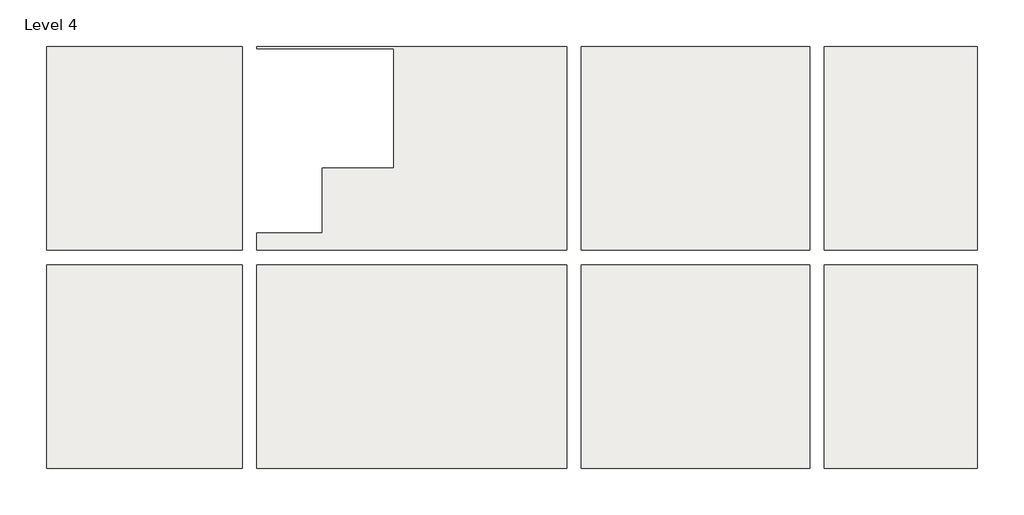
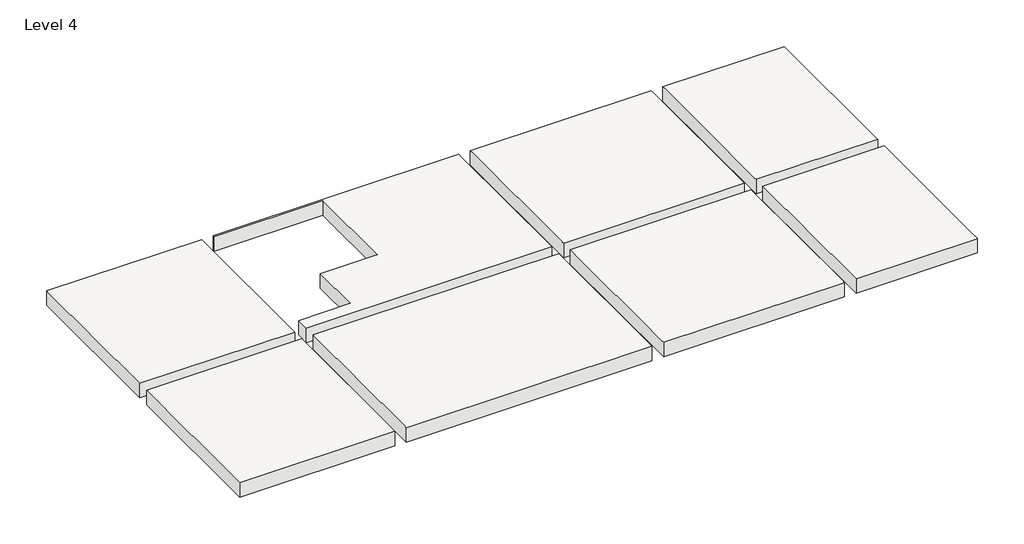
# One storey: 2 slabs.
"""IFC4 building model written with IfcOpenShell, lengths in millimetres."""

from ifc_helpers import new_model, si_unit, origin, place, context, project, spatial, faceted_brep, element, save

model = new_model("IFC4")

# Units and contexts
model_context = context("Model", 3, world=origin())
ifc_project = project(units=[si_unit("LENGTHUNIT", "METRE", prefix="MILLI")], contexts=[model_context])

# Site, building, storey
site = spatial("IfcSite", under=ifc_project)
building = spatial("IfcBuilding", under=site)
storey = spatial("IfcBuildingStorey", under=building, Name="Level 4", Elevation=6048.0)

# Slabs
placement = place(None, origin())
element("IfcSlab", 1, ObjectType="Generic 300mm", at=placement, inside=storey, context=model_context, shape_type="Brep", body=[
    faceted_brep([(-2066.1068817, 2270.4765586, 5700.0), (-5114.1068817, 2270.4765586, 5700.0), (-5114.1068817, 5445.3180792, 5700.0), (-2066.1068817, 5445.3180792, 5700.0), (-2066.1068817, 2270.4765586, 6000.0), (-2066.1068817, 2346.6765586, 6000.0), (-2066.1068817, 5407.2180792, 6000.0), (-2066.1068817, 5445.3180792, 6000.0), (-5114.1068817, 5445.3180792, 6000.0), (-5114.1068817, 5407.2180792, 6000.0), (-5114.1068817, 2346.6765586, 6000.0), (-5114.1068817, 2270.4765586, 6000.0)], [[[0, 1, 2, 3]], [[4, 5, 6, 7, 8, 9, 10, 11]], [[1, 0, 4, 11]], [[2, 1, 11, 10, 9, 8]], [[3, 2, 8, 7]], [[0, 3, 7, 6, 5, 4]]]),
])
element("IfcSlab", 2, ObjectType="Generic 300mm", at=placement, inside=storey, context=model_context, shape_type="Brep", body=[
    faceted_brep([(2988.4931183, 2270.4765586, 5700.0), (-1837.5068817, 2270.4765586, 5700.0), (-1837.5068817, 5445.3180792, 5700.0), (2988.4931183, 5445.3180792, 5700.0), (-1837.5068817, 2270.4765586, 6000.0), (2988.1931183, 2270.4765586, 6000.0), (2988.4931183, 2270.4765586, 6000.0), (2988.4931183, 2346.6765586, 6000.0), (2988.4931183, 5407.2180792, 6000.0), (2988.4931183, 5445.3180792, 6000.0), (-1837.5068817, 5445.3180792, 6000.0), (-1837.5068817, 5407.2180792, 6000.0), (-1837.5068817, 2346.6765586, 6000.0)], [[[0, 1, 2, 3]], [[4, 5, 6, 7, 8, 9, 10, 11, 12]], [[1, 0, 6, 5, 4]], [[2, 1, 4, 12, 11, 10]], [[3, 2, 10, 9]], [[0, 3, 9, 8, 7, 6]]]),
    faceted_brep([(6773.0931183, 2270.4765586, 5700.0), (3217.0931183, 2270.4765586, 5700.0), (3217.0931183, 5445.3180792, 5700.0), (6773.0931183, 5445.3180792, 5700.0), (3217.0931183, 2270.4765586, 6000.0), (6773.0931183, 2270.4765586, 6000.0), (6773.0931183, 2346.6765586, 6000.0), (6773.0931183, 5407.2180792, 6000.0), (6773.0931183, 5445.3180792, 6000.0), (3217.0931183, 5445.3180792, 6000.0), (3217.0931183, 5407.2180792, 6000.0), (3217.0931183, 2346.6765586, 6000.0)], [[[0, 1, 2, 3]], [[4, 5, 6, 7, 8, 9, 10, 11]], [[1, 0, 5, 4]], [[2, 1, 4, 11, 10, 9]], [[3, 2, 9, 8]], [[0, 3, 8, 7, 6, 5]]]),
    faceted_brep([(9389.2931183, 2270.4765586, 5700.0), (7001.6931183, 2270.4765586, 5700.0), (7001.6931183, 5445.3180792, 5700.0), (9389.2931183, 5445.3180792, 5700.0), (7001.6931183, 2270.4765586, 6000.0), (9387.3931183, 2270.4765586, 6000.0), (9389.2931183, 2270.4765586, 6000.0), (9389.2931183, 2346.6765586, 6000.0), (9389.2931183, 2354.2765586, 6000.0), (9389.2931183, 5407.2180792, 6000.0), (9389.2931183, 5445.3180792, 6000.0), (7001.6931183, 5445.3180792, 6000.0), (7001.6931183, 5407.2180792, 6000.0), (7001.6931183, 2346.6765586, 6000.0)], [[[0, 1, 2, 3]], [[4, 5, 6, 7, 8, 9, 10, 11, 12, 13]], [[1, 0, 6, 5, 4]], [[2, 1, 4, 13, 12, 11]], [[3, 2, 11, 10]], [[0, 3, 10, 9, 8, 7, 6]]]),
    faceted_brep([(7001.6931183, 5673.9180792, 5700.0), (7001.6931183, 8849.0765586, 5700.0), (9389.2931183, 8849.0765586, 5700.0), (9389.2931183, 5673.9180792, 5700.0), (7001.6931183, 8849.0765586, 6000.0), (7001.6931183, 8772.8765586, 6000.0), (7001.6931183, 5712.0180792, 6000.0), (7001.6931183, 5673.9180792, 6000.0), (9389.2931183, 5673.9180792, 6000.0), (9389.2931183, 5712.0180792, 6000.0), (9389.2931183, 8772.8765586, 6000.0), (9389.2931183, 8849.0765586, 6000.0), (9387.3931183, 8849.0765586, 6000.0)], [[[0, 1, 2, 3]], [[4, 5, 6, 7, 8, 9, 10, 11, 12]], [[1, 0, 7, 6, 5, 4]], [[2, 1, 4, 12, 11]], [[3, 2, 11, 10, 9, 8]], [[0, 3, 8, 7]]]),
    faceted_brep([(3217.0931183, 5673.9180792, 5700.0), (3217.0931183, 8849.0765586, 5700.0), (6773.0931183, 8849.0765586, 5700.0), (6773.0931183, 5673.9180792, 5700.0), (3217.0931183, 8849.0765586, 6000.0), (3217.0931183, 8772.8765586, 6000.0), (3217.0931183, 5719.6180792, 6000.0), (3217.0931183, 5712.0180792, 6000.0), (3217.0931183, 5673.9180792, 6000.0), (6773.0931183, 5673.9180792, 6000.0), (6773.0931183, 5712.0180792, 6000.0), (6773.0931183, 8772.8765586, 6000.0), (6773.0931183, 8849.0765586, 6000.0)], [[[0, 1, 2, 3]], [[4, 5, 6, 7, 8, 9, 10, 11, 12]], [[1, 0, 8, 7, 6, 5, 4]], [[2, 1, 4, 12]], [[3, 2, 12, 11, 10, 9]], [[0, 3, 9, 8]]]),
    faceted_brep([(-1837.5068817, 8849.0765586, 5700.0), (2988.4931183, 8849.0765586, 5700.0), (2988.4931183, 5673.9180792, 5700.0), (-1837.5068817, 5673.9180792, 5700.0), (-1837.5068817, 5940.7765586, 5700.0), (-821.5068817, 5940.7765586, 5700.0), (-821.5068817, 6956.7765586, 5700.0), (296.0931183, 6956.7765586, 5700.0), (296.0931183, 8810.9765586, 5700.0), (-1837.5068817, 8810.9765586, 5700.0), (2988.4931183, 8849.0765586, 6000.0), (-1837.5068817, 8849.0765586, 6000.0), (-1837.5068817, 8810.9765586, 6000.0), (296.0931183, 8810.9765586, 6000.0), (296.0931183, 6956.7765586, 6000.0), (-821.5068817, 6956.7765586, 6000.0), (-821.5068817, 5940.7765586, 6000.0), (-1837.5068817, 5940.7765586, 6000.0), (-1837.5068817, 5712.0180792, 6000.0), (-1837.5068817, 5673.9180792, 6000.0), (2988.4931183, 5673.9180792, 6000.0), (2988.4931183, 5712.0180792, 6000.0), (2988.4931183, 5719.6180792, 6000.0), (2988.4931183, 8772.8765586, 6000.0)], [[[0, 1, 2, 3, 4, 5, 6, 7, 8, 9]], [[10, 11, 12, 13, 14, 15, 16, 17, 18, 19, 20, 21, 22, 23]], [[3, 19, 18, 17, 4]], [[11, 0, 9, 12]], [[1, 0, 11, 10]], [[2, 1, 10, 23, 22, 21, 20]], [[3, 2, 20, 19]], [[5, 16, 15, 6]], [[6, 15, 14, 7]], [[7, 14, 13, 8]], [[8, 13, 12, 9]], [[16, 5, 4, 17]]]),
    faceted_brep([(-5114.1068817, 5673.9180792, 5700.0), (-5114.1068817, 8849.0765586, 5700.0), (-2066.1068817, 8849.0765586, 5700.0), (-2066.1068817, 5673.9180792, 5700.0), (-5114.1068817, 8849.0765586, 6000.0), (-5114.1068817, 8772.8765586, 6000.0), (-5114.1068817, 5712.0180792, 6000.0), (-5114.1068817, 5673.9180792, 6000.0), (-2066.1068817, 5673.9180792, 6000.0), (-2066.1068817, 5712.0180792, 6000.0), (-2066.1068817, 8772.8765586, 6000.0), (-2066.1068817, 8849.0765586, 6000.0)], [[[0, 1, 2, 3]], [[4, 5, 6, 7, 8, 9, 10, 11]], [[1, 0, 7, 6, 5, 4]], [[2, 1, 4, 11]], [[3, 2, 11, 10, 9, 8]], [[0, 3, 8, 7]]]),
])

save(model, "model.ifc")

# Revit data of these elements
# Type "Generic 300mm"
#   Function = 0
#   Layers, outside or top first: 300 mm no material (function 1)
# Elements 1, 2 (IfcSlab, "Generic 300mm")
#   Height Offset From Level = -48 mm
#   built-in parameter 1001954 = 1
#   Phase Created = New Construction
#   Materials on its faces: "Default Floor"
# Materials
#   "Default Floor": colour RGB 127 127 127, transparency 0, Cost = 0
